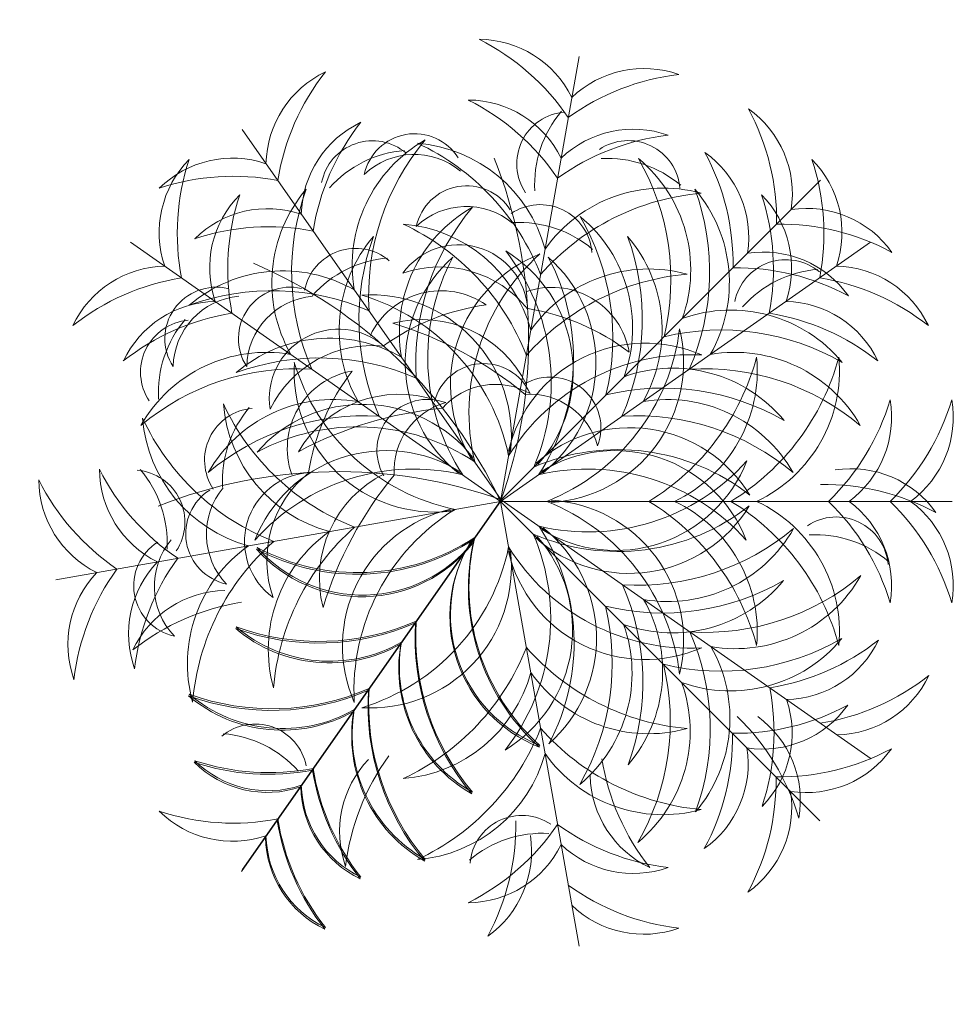
# Model space of a CAD drawing. Units: inches. Extents: x -48 to 50072, y 0 to 21068.
# Tile 41 of 75: x 493 to 519, y 306 to 334. Entities that reach past the tile are written whole.
import ezdxf

# ---------------------------------------------------------------- set-up
doc = ezdxf.new("R2010")
doc.units = ezdxf.units.IN
doc.header["$MEASUREMENT"] = 0
doc.layers.add('A-ANNO-DIMS', color=2, linetype='Continuous', lineweight=18)
doc.layers.add('L-PLNT', color=94, linetype='Continuous', lineweight=13)
doc.styles.get("Standard").update_dxf_attribs({"font": 'arial.ttf'})
doc.dimstyles.get("Standard").update_dxf_attribs({"dimtxt": 8, "dimasz": 0.18, "dimexe": 0.18, "dimexo": 0.0625, "dimgap": 0.09, "dimtad": 0, "dimtih": 1, "dimtoh": 1, "dimdec": 1, "dimzin": 0, "dimdsep": 46, "dimlunit": 4, "dimtxsty": 'Standard', "dimblk": 'ARCHTICK', "dimcen": 0.09, "dimadec": 0, "dimazin": 0, "dimtfac": 1, "dimtdec": 1, "dimtofl": 0, "dimtmove": 0, "dimatfit": 3, "dimldrblk": 'ARCHTICK', "dimfxl": 1, "dimtolj": 1, "dimtzin": 0, "dimarcsym": 0})

# ---------------------------------------------------------------- blocks, each defined once
blk = doc.blocks.new('A$C5D061C3B')
for p, q in [((3.3772, 6.6792), (3.3772, 3.3772)), ((1.4832, 6.082), (3.3772, 3.3772)), ((5.2591, 6.0863), (3.3651, 3.3814)), ((1.0302, 5.7163), (3.3651, 3.3814)), ((5.712, 5.712), (3.3772, 3.3772)), ((0.1253, 3.9506), (3.3772, 3.3772)), ((6.629, 3.9506), (3.3772, 3.3772)), ((0.6603, 1.4875), (3.3651, 3.3814)), ((1.4832, 0.6723), (3.3772, 3.3772)), ((6.0699, 1.4875), (3.3651, 3.3814)), ((3.9506, 0.1253), (3.3772, 3.3772)), ((6.082, 1.4832), (3.3772, 3.3772))]:
    blk.add_line(p, q)
for centre, radius, start, end in [((2.7629, 5.9242), 0.7621, 36.28997, 99.62433), ((2.1448, 5.0319), 1.7154, 44.07628, 73.37936), ((3.9915, 5.9242), 0.7621, 80.37567, 143.71003), ((4.6096, 5.0319), 1.7154, 106.62064, 135.92372), ((3.9007, 5.9388), 0.7621, 125.37567, 188.71003), ((4.9688, 5.7448), 1.7154, 151.62064, 180.92372), ((2.4194, 5.816), 0.7621, 115.37567, 178.71003), ((3.4376, 5.4395), 1.7154, 141.62064, 170.92372), ((3.3047, 5.4438), 1.7154, 9.07628, 38.37936), ((4.3228, 5.8202), 0.7621, 1.28997, 64.62433), ((1.9984, 5.6169), 0.7621, 125.37567, 188.71003), ((3.0665, 5.4229), 1.7154, 151.62064, 180.92372), ((2.7629, 5.4738), 0.7621, 36.28997, 99.62433), ((2.1448, 4.5814), 1.7154, 44.07628, 73.37936), ((3.9915, 5.4738), 0.7621, 80.37567, 143.71003), ((4.6096, 4.5814), 1.7154, 106.62064, 135.92372), ((3.8712, 5.8319), 0.3799, 94.742, 213.74753), ((4.4474, 5.6807), 0.826, 139.61802, 183.21064), ((4.7438, 5.6126), 0.7621, 351.28997, 54.62433), ((3.6758, 5.4187), 1.7154, 359.07628, 28.37936), ((2.6778, 5.4469), 0.7621, 115.37567, 178.71003), ((3.696, 5.0705), 1.7154, 141.62064, 170.92372), ((4.0645, 5.4512), 0.7621, 1.28997, 64.62433), ((3.0463, 5.0747), 1.7154, 9.07628, 38.37936), ((3.3438, 5.0894), 1.0556, 119.60629, 189.75109), ((4.1771, 4.8688), 1.7695, 139.96343, 183.62881), ((3.3985, 5.0936), 1.0556, 350.24891, 60.39371), ((2.5652, 4.8731), 1.7695, 356.37119, 40.03657), ((2.317, 5.2983), 0.7621, 125.37567, 188.71003), ((3.385, 5.1044), 1.7154, 151.62064, 180.92372), ((3.3573, 5.1001), 1.7154, 359.07628, 28.37936), ((4.4253, 5.2941), 0.7621, 351.28997, 54.62433), ((1.413, 5.1113), 0.7621, 71.28997, 134.62433), ((3.0349, 5.0618), 1.0556, 129.60629, 199.75109), ((3.8939, 4.9893), 1.7695, 149.96343, 193.62881), ((2.4224, 4.7989), 1.0556, 25.24891, 95.39371), ((1.8663, 4.1402), 1.7695, 31.37119, 75.03657), ((4.3319, 4.7989), 1.0556, 84.60629, 154.75109), ((4.888, 4.1402), 1.7695, 104.96343, 148.62881), ((2.8484, 4.9851), 1.7695, 346.37119, 30.03657), ((3.7074, 5.0576), 1.0556, 340.24891, 50.39371), ((1.4185, 4.0258), 1.7154, 79.07628, 108.37936), ((1.9907, 5.4623), 0.3799, 139.742, 258.74753), ((2.5051, 5.7628), 0.826, 184.61802, 228.21064), ((5.5642, 4.8068), 0.7621, 80.37567, 143.71003), ((6.1823, 3.9144), 1.7154, 106.62064, 135.92372), ((1.1297, 4.7481), 0.7621, 81.28997, 144.62433), ((1.6714, 4.7422), 0.7621, 71.28997, 134.62433), ((3.6883, 4.5973), 1.0556, 119.60629, 189.75109), ((4.5216, 4.3768), 1.7695, 139.96343, 183.62881), ((2.2207, 4.3811), 1.7695, 356.37119, 40.03657), ((3.054, 4.6016), 1.0556, 350.24891, 60.39371), ((5.0709, 4.7465), 0.7621, 45.37567, 108.71003), ((5.6126, 4.7438), 0.7621, 35.37567, 98.71003), ((3.4596, 4.6371), 1.0556, 129.60629, 199.75109), ((4.3186, 4.5646), 1.7695, 149.96343, 193.62881), ((3.2827, 4.6328), 1.0556, 340.24891, 50.39371), ((2.4237, 4.5604), 1.7695, 346.37119, 30.03657), ((1.3236, 3.68), 1.7154, 89.07628, 118.37936), ((1.6769, 3.6567), 1.7154, 79.07628, 108.37936), ((5.0653, 3.661), 1.7154, 71.62064, 100.92372), ((5.4187, 3.6758), 1.7154, 61.62064, 90.92372), ((2.4224, 4.1982), 1.0556, 25.24891, 95.39371), ((4.3319, 4.1982), 1.0556, 84.60629, 154.75109), ((1.4482, 4.4296), 0.7621, 81.28997, 144.62433), ((1.8663, 3.5396), 1.7695, 31.37119, 75.03657), ((3.8676, 4.3207), 1.029, 121.36542, 221.57406), ((4.5556, 4.2369), 1.5567, 141.81221, 203.33354), ((4.888, 3.5396), 1.7695, 104.96343, 148.62881), ((2.1867, 4.2327), 1.5567, 336.66646, 38.18779), ((2.8746, 4.3165), 1.029, 318.42594, 58.63458), ((5.2941, 4.4253), 0.7621, 35.37567, 98.71003), ((4.0352, 4.215), 1.029, 111.36542, 211.57406), ((2.7071, 4.2192), 1.029, 328.42594, 68.63458), ((2.0441, 4.0172), 1.5567, 346.66646, 48.18779), ((4.6982, 4.0129), 1.5567, 131.81221, 193.33354), ((1.6421, 3.3615), 1.7154, 89.07628, 118.37936), ((1.7796, 3.9941), 1.0556, 60.24891, 130.39371), ((4.9626, 3.9984), 1.0556, 49.60629, 119.75109), ((5.1001, 3.3573), 1.7154, 61.62064, 90.92372), ((1.7019, 3.1357), 1.7695, 66.37119, 110.03657), ((5.0404, 3.1399), 1.7695, 69.96343, 113.62881), ((2.1429, 4.5643), 1.0556, 164.60629, 234.75109), ((2.888, 4.9976), 1.7695, 184.96343, 228.62881), ((3.25, 4.4348), 1.029, 156.36542, 256.57406), ((3.8617, 4.7608), 1.5567, 176.81221, 238.33354), ((2.8927, 4.7608), 1.5567, 301.66646, 3.18779), ((3.5043, 4.4348), 1.029, 283.42594, 23.63458), ((3.8663, 4.9976), 1.7695, 311.37119, 355.03657), ((4.6115, 4.5643), 1.0556, 305.24891, 15.39371), ((1.6847, 3.7116), 1.0556, 70.24891, 140.39371), ((5.0576, 3.7074), 1.0556, 39.60629, 109.75109), ((0.9755, 4.4244), 0.7621, 160.37567, 223.71003), ((1.9616, 4.8782), 1.7154, 186.62064, 215.92372), ((1.1202, 4.3101), 0.3799, 94.742, 213.74753), ((1.6965, 4.1589), 0.826, 139.61802, 183.21064), ((2.7344, 4.46), 1.0556, 164.60629, 234.75109), ((3.4796, 4.8933), 1.7695, 184.96343, 228.62881), ((2.3576, 3.686), 1.029, 3.42594, 103.63458), ((1.9304, 3.1403), 1.5567, 21.66646, 83.18779), ((4.3967, 3.686), 1.029, 76.36542, 176.57406), ((4.8239, 3.1403), 1.5567, 96.81221, 158.33354), ((3.2748, 4.8933), 1.7695, 311.37119, 355.03657), ((4.02, 4.46), 1.0556, 305.24891, 15.39371), ((4.7927, 4.8782), 1.7154, 324.07628, 353.37936), ((5.7789, 4.4244), 0.7621, 316.28997, 19.62433), ((1.7572, 2.8527), 1.7695, 76.37119, 120.03657), ((4.9851, 2.8484), 1.7695, 59.96343, 103.62881), ((1.4191, 4.3462), 0.7621, 160.37567, 223.71003), ((2.4052, 4.8), 1.7154, 186.62064, 215.92372), ((2.1242, 3.5021), 1.0556, 60.24891, 130.39371), ((4.6181, 3.5064), 1.0556, 49.60629, 119.75109), ((4.3491, 4.8), 1.7154, 324.07628, 353.37936), ((5.3352, 4.3462), 0.7621, 316.28997, 19.62433), ((4.9885, 5.8124), 1.7154, 279.07628, 308.37936), ((5.3649, 4.7942), 0.7621, 271.28997, 334.62433), ((2.0464, 2.6436), 1.7695, 66.37119, 110.03657), ((4.6959, 2.6479), 1.7695, 69.96343, 113.62881), ((2.1094, 3.2869), 1.0556, 70.24891, 140.39371), ((4.6328, 3.2827), 1.0556, 39.60629, 109.75109), ((2.3872, 3.7525), 0.574, 99.98654, 199.40339), ((3.5988, 3.3144), 1.651, 142.57587, 170.89417), ((2.1819, 2.428), 1.7695, 76.37119, 120.03657), ((4.5604, 2.4237), 1.7695, 59.96343, 103.62881), ((2.8402, 3.7391), 0.3717, 69.22575, 210.12788), ((1.5885, 3.6663), 0.3799, 94.742, 213.74753), ((2.1647, 3.515), 0.826, 139.61802, 183.21064), ((2.3649, 3.0454), 1.029, 38.42594, 138.63458), ((3.1091, 3.5901), 0.5151, 105.43977, 183.66943), ((4.3774, 3.0496), 1.029, 41.36542, 141.57406), ((0.7621, 3.2145), 0.7621, 116.28997, 179.62433), ((2.4258, 2.8789), 1.029, 48.42594, 148.63458), ((2.3279, 2.3533), 1.5567, 56.66646, 118.18779), ((4.4143, 2.3575), 1.5567, 61.81221, 123.33354), ((4.3165, 2.8746), 1.029, 31.36542, 131.57406), ((1.5336, 2.4508), 1.7154, 124.07628, 153.37936), ((1.2058, 3.1363), 0.7621, 116.28997, 179.62433), ((1.0616, 4.4517), 0.826, 229.61802, 273.21064), ((0.9103, 3.8754), 0.3799, 184.742, 303.74753), ((5.5486, 3.1363), 0.7621, 0.37567, 63.71003), ((1.9772, 2.3726), 1.7154, 124.07628, 153.37936), ((2.5096, 2.1909), 1.5567, 66.66646, 128.18779), ((4.2327, 2.1867), 1.5567, 51.81221, 113.33354), ((6.0526, 3.5327), 0.3799, 146.25247, 265.258), ((4.7771, 2.3726), 1.7154, 26.62064, 55.92372), ((1.8113, 2.6838), 1.0556, 105.24891, 175.39371), ((4.9431, 2.6838), 1.0556, 4.60629, 74.75109), ((6.6289, 3.6839), 0.826, 176.78936, 220.38198), ((2.3633, 2.0218), 1.7695, 111.37119, 155.03657), ((2.7293, 4.7024), 1.5567, 221.81221, 283.33354), ((2.5273, 4.0394), 1.029, 201.36542, 301.57406), ((4.0009, 4.7024), 1.5567, 256.66646, 318.18779), ((4.0129, 4.6982), 1.5567, 256.66646, 318.18779), ((4.2029, 4.0394), 1.029, 238.42594, 338.63458), ((4.215, 4.0352), 1.029, 238.42594, 338.63458), ((4.391, 2.0218), 1.7695, 24.96343, 68.62881), ((5.9345, 2.8416), 0.7621, 35.37567, 98.71003), ((2.1851, 0.015), 3.5672, 70.47721, 111.6585), ((2.4028, 2.5795), 1.0556, 105.24891, 175.39371), ((2.9548, 1.9175), 1.7695, 111.37119, 155.03657), ((2.0067, 3.0714), 0.5057, 93.87442, 233.97626), ((2.4891, 2.9324), 0.8252, 128.75364, 199.09705), ((2.9034, 2.8005), 0.8553, 116.44767, 194.36723), ((4.7443, 1.7792), 2.7893, 140.40074, 163.13904), ((2.7415, 3.2534), 0.3717, 114.22575, 255.12788), ((3.0371, 3.3382), 0.5151, 150.43977, 228.66943), ((3.7995, 1.9175), 1.7695, 24.96343, 68.62881), ((4.3515, 2.5795), 1.0556, 4.60629, 74.75109), ((1.7505, 3.1258), 0.5286, 140.18449, 223.65396), ((2.896, 2.4268), 1.029, 83.42594, 183.63458), ((3.8584, 2.4268), 1.029, 356.36542, 96.57406), ((5.7406, 1.7735), 1.7154, 61.62064, 90.92372), ((1.4473, 3.129), 0.3765, 122.05775, 257.85325), ((3.3592, 1.9113), 1.5567, 101.66646, 163.18779), ((3.3951, 1.9113), 1.5567, 16.81221, 78.33354), ((4.9116, 0.1568), 3.5672, 115.47721, 156.6585), ((6.7273, 2.1893), 3.5672, 160.47721, 201.6585), ((2.4118, 2.9425), 0.574, 144.98654, 244.40339), ((3.5783, 3.4895), 1.651, 187.57587, 215.89417), ((2.1449, 3.6925), 1.0556, 209.60629, 279.75109), ((2.3655, 4.5259), 1.7695, 229.96343, 273.62881), ((3.6969, 2.3691), 1.029, 128.42594, 228.63458), ((4.389, 2.3322), 1.5567, 146.66646, 208.18779), ((2.3412, 2.3322), 1.5567, 331.81221, 33.33354), ((2.3533, 2.3279), 1.5567, 331.81221, 33.33354), ((3.0333, 2.3691), 1.029, 311.36542, 51.57406), ((3.0454, 2.3649), 1.029, 311.36542, 51.57406), ((4.3647, 4.5259), 1.7695, 266.37119, 310.03657), ((4.3768, 4.5216), 1.7695, 266.37119, 310.03657), ((4.5853, 3.6925), 1.0556, 260.24891, 330.39371), ((4.5973, 3.6883), 1.0556, 260.24891, 330.39371), ((2.3279, 4.401), 1.5567, 241.81221, 303.33354), ((4.6982, 2.7414), 1.5567, 166.66646, 228.18779), ((1.0668, 2.7485), 0.3765, 122.05775, 257.85325), ((1.3701, 2.7454), 0.5286, 140.18449, 223.65396), ((2.3649, 3.7089), 1.029, 221.36542, 321.57406), ((1.9113, 3.3592), 1.5567, 286.81221, 348.33354), ((4.0352, 2.5394), 1.029, 148.42594, 248.63458), ((4.7608, 3.8617), 1.5567, 211.66646, 273.18779), ((2.4268, 2.896), 1.029, 266.36542, 6.57406), ((3.0031, 2.8444), 0.3717, 159.22575, 300.12788), ((3.1522, 3.1134), 0.5151, 195.43977, 273.66943), ((5.4738, 3.2139), 2.7893, 185.40074, 208.13904), ((4.4348, 3.25), 1.029, 193.42594, 293.63458), ((3.45, 2.6344), 0.8553, 161.44767, 239.36723), ((1.8734, 4.1813), 1.7695, 229.96343, 273.62881), ((1.6529, 3.348), 1.0556, 209.60629, 279.75109), ((4.8568, 4.1813), 1.7695, 266.37119, 310.03657), ((4.8688, 4.1771), 1.7695, 266.37119, 310.03657), ((5.0773, 3.348), 1.0556, 260.24891, 330.39371), ((5.0894, 3.3438), 1.0556, 260.24891, 330.39371), ((4.0986, 2.0506), 1.7695, 156.37119, 200.03657), ((2.6316, 2.0506), 1.7695, 339.96343, 23.62881), ((2.6436, 2.0464), 1.7695, 339.96343, 23.62881), ((1.1216, 2.4409), 0.3799, 139.742, 258.74753), ((1.636, 2.7415), 0.826, 184.61802, 228.21064), ((3.2401, 2.1284), 1.0556, 150.24891, 220.39371), ((4.9631, 4.7486), 2.7893, 230.40074, 253.13904), ((3.4901, 2.1284), 1.0556, 319.60629, 29.75109), ((3.5021, 2.1242), 1.0556, 319.60629, 29.75109), ((1.9079, 2.3168), 0.3799, 139.742, 258.74753), ((2.4223, 2.6173), 0.826, 184.61802, 228.21064), ((2.6243, 2.1919), 0.5057, 138.87442, 278.97626), ((3.0637, 2.4347), 0.8252, 173.75364, 244.09705), ((3.9418, 2.9077), 0.8553, 206.44767, 284.36723), ((6.244, 3.9482), 1.7154, 234.07628, 263.37936), ((2.0464, 4.1107), 1.7695, 249.96343, 293.62881), ((2.1242, 3.2522), 1.0556, 229.60629, 299.75109), ((4.5216, 2.3775), 1.7695, 176.37119, 220.03657), ((3.6066, 1.7061), 1.7695, 156.37119, 200.03657), ((3.1236, 1.7061), 1.7695, 339.96343, 23.62881), ((3.1357, 1.7019), 1.7695, 339.96343, 23.62881), ((5.7902, 2.9621), 0.7621, 226.28997, 289.62433), ((1.6718, 3.7002), 1.7154, 231.62064, 260.92372), ((1.2953, 2.6821), 0.7621, 205.37567, 268.71003), ((2.7481, 1.7839), 1.0556, 150.24891, 220.39371), ((3.6883, 2.157), 1.0556, 170.24891, 240.39371), ((1.9175, 2.9548), 1.7695, 294.96343, 338.62881), ((4.8933, 3.4796), 1.7695, 221.37119, 265.03657), ((3.9821, 1.7839), 1.0556, 319.60629, 29.75109), ((3.9941, 1.7796), 1.0556, 319.60629, 29.75109), ((5.0584, 3.7002), 1.7154, 279.07628, 308.37936), ((5.0705, 3.696), 1.7154, 279.07628, 308.37936), ((5.4349, 2.6821), 0.7621, 271.28997, 334.62433), ((5.4469, 2.6778), 0.7621, 271.28997, 334.62433), ((3.4279, 3.6031), 1.651, 232.57587, 260.89417), ((2.9898, 2.3915), 0.574, 189.98654, 289.40339), ((0.9263, 2.4237), 0.7621, 205.37567, 268.71003), ((1.3028, 3.4418), 1.7154, 231.62064, 260.92372), ((2.5795, 2.4028), 1.0556, 274.60629, 344.75109), ((4.46, 2.7344), 1.0556, 215.24891, 285.39371), ((5.4274, 3.4418), 1.7154, 279.07628, 308.37936), ((5.4395, 3.4376), 1.7154, 279.07628, 308.37936), ((5.8039, 2.4237), 0.7621, 271.28997, 334.62433), ((5.816, 2.4194), 0.7621, 271.28997, 334.62433), ((1.7019, 3.6187), 1.7695, 249.96343, 293.62881), ((1.7796, 2.7602), 1.0556, 229.60629, 299.75109), ((3.0855, 1.6812), 1.7154, 169.07628, 198.37936), ((2.4047, 2.0492), 0.5286, 185.18449, 268.65396), ((4.1771, 1.8855), 1.7695, 176.37119, 220.03657), ((3.8099, 2.4933), 0.8252, 218.75364, 289.09705), ((3.6709, 2.011), 0.5057, 183.87442, 323.97626), ((5.3845, 1.5838), 0.3799, 101.25247, 220.258), ((3.6447, 1.6812), 1.7154, 341.62064, 10.92372), ((3.6567, 1.6769), 1.7154, 341.62064, 10.92372), ((2, 1.6757), 0.7621, 161.28997, 224.62433), ((2.188, 1.837), 0.3765, 167.05775, 302.85325), ((5.8989, 1.2832), 0.826, 131.78936, 175.38198), ((4.7302, 1.6757), 0.7621, 315.37567, 18.71003), ((4.7422, 1.6714), 0.7621, 315.37567, 18.71003), ((3.3438, 1.665), 1.0556, 170.24891, 240.39371), ((2.7165, 1.4228), 1.7154, 169.07628, 198.37936), ((4.0137, 1.4228), 1.7154, 341.62064, 10.92372), ((1.631, 1.4173), 0.7621, 161.28997, 224.62433), ((2.0218, 2.3633), 1.7695, 294.96343, 338.62881), ((4.9976, 2.888), 1.7695, 221.37119, 265.03657), ((5.0992, 1.4173), 0.7621, 315.37567, 18.71003), ((3.2272, 2.169), 0.826, 229.61802, 273.21064), ((3.076, 1.5927), 0.3799, 184.742, 303.74753), ((2.6838, 1.8113), 1.0556, 274.60629, 344.75109), ((4.5643, 2.1429), 1.0556, 215.24891, 285.39371), ((1.6714, 2.0121), 0.7621, 225.37567, 288.71003), ((1.6769, 3.0976), 1.7154, 251.62064, 280.92372), ((2.4047, 1.5112), 0.5286, 185.18449, 268.65396), ((5.8081, 1.7538), 1.7154, 189.07628, 218.37936), ((2.188, 1.299), 0.3765, 167.05775, 302.85325), ((3.696, 1.6838), 1.7154, 189.07628, 218.37936), ((3.6165, 1.7548), 0.5286, 230.18449, 313.65396), ((3.6133, 1.4515), 0.3765, 212.05775, 347.85325), ((4.79, 1.3774), 0.7621, 181.28997, 244.62433), ((2.6778, 1.3074), 0.7621, 181.28997, 244.62433), ((1.4185, 2.7286), 1.7154, 251.62064, 280.92372), ((1.413, 1.6431), 0.7621, 225.37567, 288.71003), ((2.4322, 1.1245), 0.3799, 184.742, 303.74753), ((3.4376, 1.3148), 1.7154, 189.07628, 218.37936), ((2.5834, 1.7007), 0.826, 229.61802, 273.21064), ((2.3726, 1.9772), 1.7154, 296.62064, 325.92372), ((3.5285, 0.6896), 0.3799, 56.25247, 175.258), ((4.8, 2.4052), 1.7154, 234.07628, 263.37936), ((3.6797, 0.1134), 0.826, 86.78936, 130.38198), ((3.9969, 1.3743), 0.5286, 230.18449, 313.65396), ((3.9938, 1.0711), 0.3765, 212.05775, 347.85325), ((2.4194, 0.9384), 0.7621, 181.28997, 244.62433), ((3.1363, 1.2058), 0.7621, 270.37567, 333.71003), ((4.3462, 1.4191), 0.7621, 226.28997, 289.62433), ((2.4508, 1.5336), 1.7154, 296.62064, 325.92372), ((4.8782, 1.9616), 1.7154, 234.07628, 263.37936), ((3.2145, 0.7621), 0.7621, 270.37567, 333.71003), ((4.4244, 0.9755), 0.7621, 226.28997, 289.62433)]:
    blk.add_arc(centre, radius, start, end)
blk = doc.blocks.new('_ArchTick')
at = {"color": 0, "linetype": 'ByBlock', "const_width": 0.15}
blk.add_lwpolyline([(-0.5, -0.5), (0.5, 0.5)], dxfattribs=at)
blk = doc.blocks.new('*D119')
at = {"layer": 'A-ANNO-DIMS', "color": 0, "lineweight": -2, "transparency": 16777216}
for p, q in [((463.517, 451.012), (463.517, 165.945)), ((549.017, 451.012), (549.017, 165.945)), ((463.517, 166.125), (495.752, 166.125)), ((549.017, 166.125), (516.783, 166.125))]:
    blk.add_line(p, q, dxfattribs=at)
at = {"layer": 'Defpoints', "color": 0, "transparency": 16777216}
for p in [(463.517, 451.075), (549.017, 451.075), (549.017, 166.125)]:
    blk.add_point(p, dxfattribs=at)
at = {"layer": 'A-ANNO-DIMS', "color": 0, "lineweight": -2, "transparency": 16777216, "xscale": 0.18, "yscale": 0.18, "zscale": 0.18, "rotation": 180}
blk.add_blockref('_ArchTick', (463.517, 166.125), dxfattribs=at)
at = {"layer": 'A-ANNO-DIMS', "color": 0, "lineweight": -2, "transparency": 16777216, "xscale": 0.18, "yscale": 0.18, "zscale": 0.18}
blk.add_blockref('_ArchTick', (549.017, 166.125), dxfattribs=at)
at = {"layer": 'A-ANNO-DIMS', "color": 0, "transparency": 16777216, "insert": (506.267, 166.125), "char_height": 8, "attachment_point": 5}
blk.add_mtext('\\A1;85.5', dxfattribs=at)

msp = doc.modelspace()

# ---------------------------------------------------------------- block references
at = {"layer": 'L-PLNT', "xscale": 3.862191520948588, "yscale": 3.862191520948588, "zscale": 3.862191520948588, "rotation": 270}
msp.add_blockref('A$C5D061C3B', (493.073, 333.124), dxfattribs=at)

# ---------------------------------------------------------------- dimensions: what is measured, and where the dimension line sits
at = {"layer": 'A-ANNO-DIMS'}
dim = msp.add_linear_dim(base=(549.017, 166.125), p1=(463.517, 451.075), p2=(549.017, 451.075), dimstyle='Standard', override={"dimdec": 1, "dimlfac": 1, "dimrnd": 0, "dimzin": 0, "dimdsep": 46, "dimlunit": 2}, dxfattribs=at)
dim.commit()
dim.dimension.update_dxf_attribs({"geometry": '*D119', "text_midpoint": (506.267, 166.125)})

doc.saveas('drawing.dxf')
